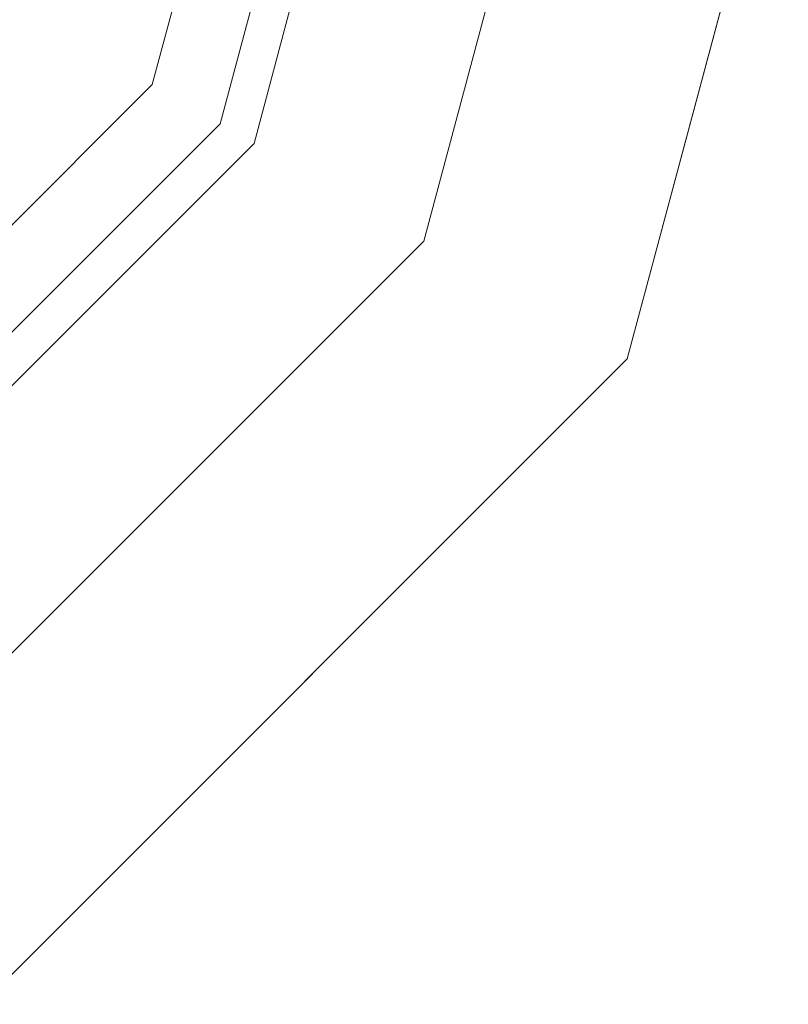
# Model space of a CAD drawing. Units: inches. Extents: x 375 to 1122, y 27 to 1069.
# Tile 118 of 155: x 715.443 to 717.857, y 890.318 to 893.412. Entities that reach past the tile are written whole.
import ezdxf

# ---------------------------------------------------------------- set-up
doc = ezdxf.new("R2010")
doc.units = ezdxf.units.IN
doc.layers.add('Furniture', color=30, linetype='Continuous', lineweight=18)

# ---------------------------------------------------------------- blocks, each defined once
blk = doc.blocks.new('A$C403C54AD')
at = {"linetype": 'ByBlock', "invisible_edges": 5}
for points in [[(1.149468, 0.81008, -0.008737), (1.140233, 0.794084, -0.008737), (1.080205, 0.810169, -0.008737), (1.080205, 0.828639, -0.008737)], [(1.132537, 0.780755, -0.02259), (1.149468, 0.81008, -0.013355), (1.080205, 0.828639, -0.013355), (1.080205, 0.794777, -0.02259)], [(1.140233, 0.794084, -0.008737), (1.130998, 0.778089, -0.014894), (1.080205, 0.791699, -0.014894), (1.080205, 0.810169, -0.008737)], [(1.170847, 0.742445, -0.02259), (1.200173, 0.759376, -0.013355), (1.149468, 0.81008, -0.013355), (1.132537, 0.780755, -0.02259)], [(1.200173, 0.759376, -0.008737), (1.184177, 0.750141, -0.008737), (1.140233, 0.794084, -0.008737), (1.149468, 0.81008, -0.008737)], [(1.12792, 0.772757, -0.031825), (1.132537, 0.780755, -0.02259), (1.080205, 0.794777, -0.02259), (1.080205, 0.785542, -0.031825)], [(1.184177, 0.750141, -0.008737), (1.168181, 0.740905, -0.014894), (1.130998, 0.778089, -0.014894), (1.140233, 0.794084, -0.008737)], [(1.130998, 0.778089, -0.014894), (1.080205, 0.690112, -0.014894), (1.080205, 0.690112, -0.014894), (1.080205, 0.791699, -0.014894)], [(1.162849, 0.737827, -0.031825), (1.170847, 0.742445, -0.02259), (1.132537, 0.780755, -0.02259), (1.12792, 0.772757, -0.031825)], [(1.168181, 0.740905, -0.014894), (1.080205, 0.690112, -0.014894), (1.080205, 0.690112, -0.014894), (1.130998, 0.778089, -0.014894)]]:
    blk.add_3dface(points, dxfattribs=at)
at = {"linetype": 'ByBlock'}
for points in [[(1.149468, 0.81008, -0.013355), (1.149468, 0.81008, -0.008737), (1.080205, 0.828639, -0.008737), (1.080205, 0.828639, -0.013355)], [(1.200173, 0.759376, -0.013355), (1.200173, 0.759376, -0.008737), (1.149468, 0.81008, -0.008737), (1.149468, 0.81008, -0.013355)]]:
    blk.add_3dface(points, dxfattribs=at)

msp = doc.modelspace()

# ---------------------------------------------------------------- block references
at = {"layer": 'Furniture', "xscale": 39.9918517141215, "yscale": 39.9918517141215, "zscale": 39.9918517141215, "rotation": 270}
msp.add_blockref('A$C403C54AD', (684.9549, 938.3156, 0.024), dxfattribs=at)

doc.saveas('drawing.dxf')
